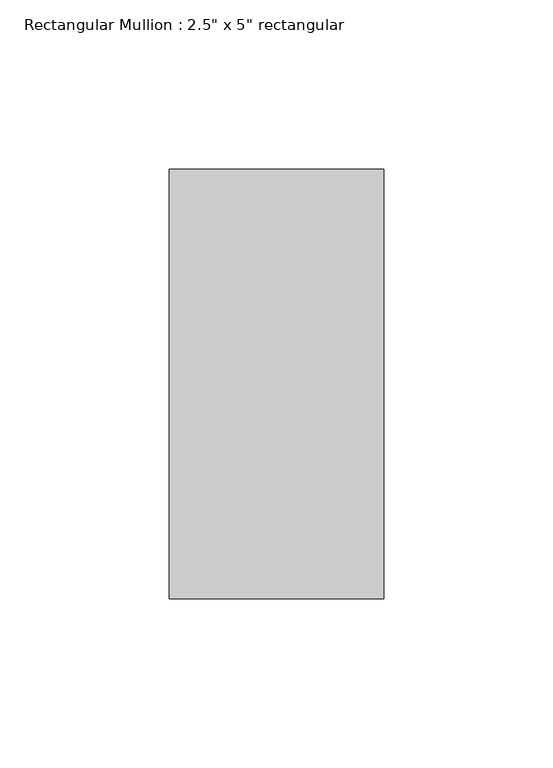
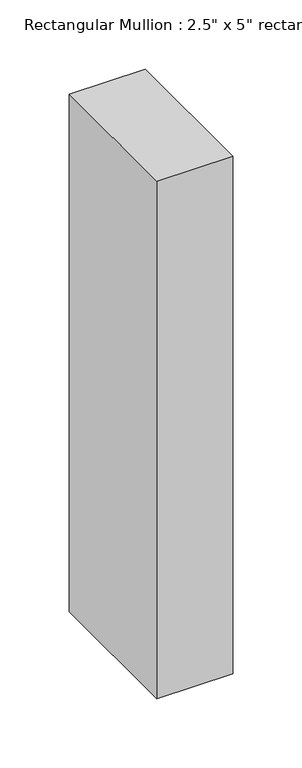
"""IFC4 building model written with IfcOpenShell, lengths in millimetres: member geometry."""

from ifc_helpers import new_model, si_unit, frame, origin, place, context, project, spatial, polyline, outline, extrude, source, transform, mapped, element, save


def member_15823cb3(model_context):
    return source(origin(), model_context, "Body", "SweptSolid", [
        extrude(outline(polyline([(0.0, 63.5), (0.0, -63.5), (-63.5, -63.5), (-63.5, 63.5), (0.0, 63.5)])), frame((0.0, 0.0, -457.2), z_axis=(0.0, 0.0, 1.0), x_axis=(1.0, 0.0, 0.0)), (0.0, 0.0, 1.0), 457.2),
    ])


if __name__ == "__main__":
    model = new_model("IFC4")
    model_context = context("Model", 3, world=origin())
    ifc_project = project(units=[si_unit("LENGTHUNIT", "METRE", prefix="MILLI")], contexts=[model_context])
    site = spatial("IfcSite", under=ifc_project)
    building = spatial("IfcBuilding", under=site)
    placement = place(None, origin())
    member_shape = member_15823cb3(model_context)
    element("IfcMember", 1, ObjectType="Rectangular Mullion : 2.5\" x 5\" rectangular", at=placement, inside=building, context=model_context, shape_type="MappedRepresentation", body=[
        mapped(member_shape, transform((0.0, 0.0, 0.0), x_axis=(1.0, 0.0, 0.0), y_axis=(0.0, 1.0, 0.0), z_axis=(0.0, 0.0, 1.0))),
    ])
    save(model, "model.ifc")

# Revit data of these elements
# Type "Rectangular Mullion : 2.5\" x 5\" rectangular"
#   built-in parameter 1007304 = 0.416667 (stored number, unit not read)
#   built-in parameter 1007301 = 0.104167 (stored number, unit not read)
#   built-in parameter 1007300 = 0.104167 (stored number, unit not read)
